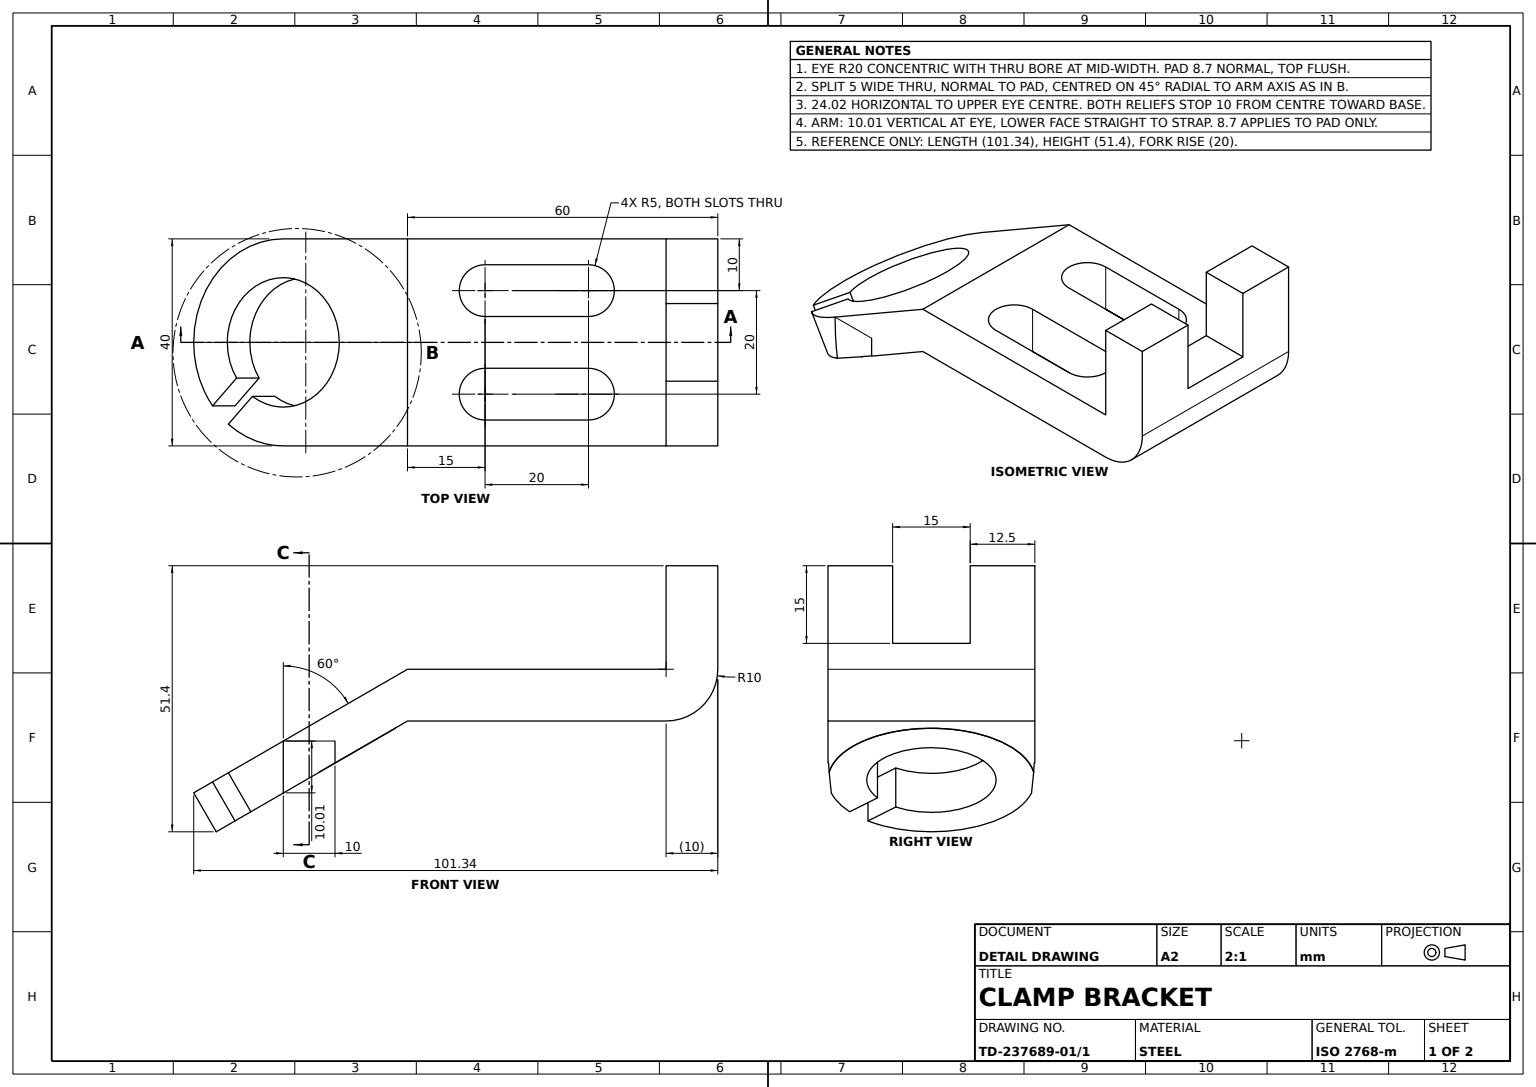
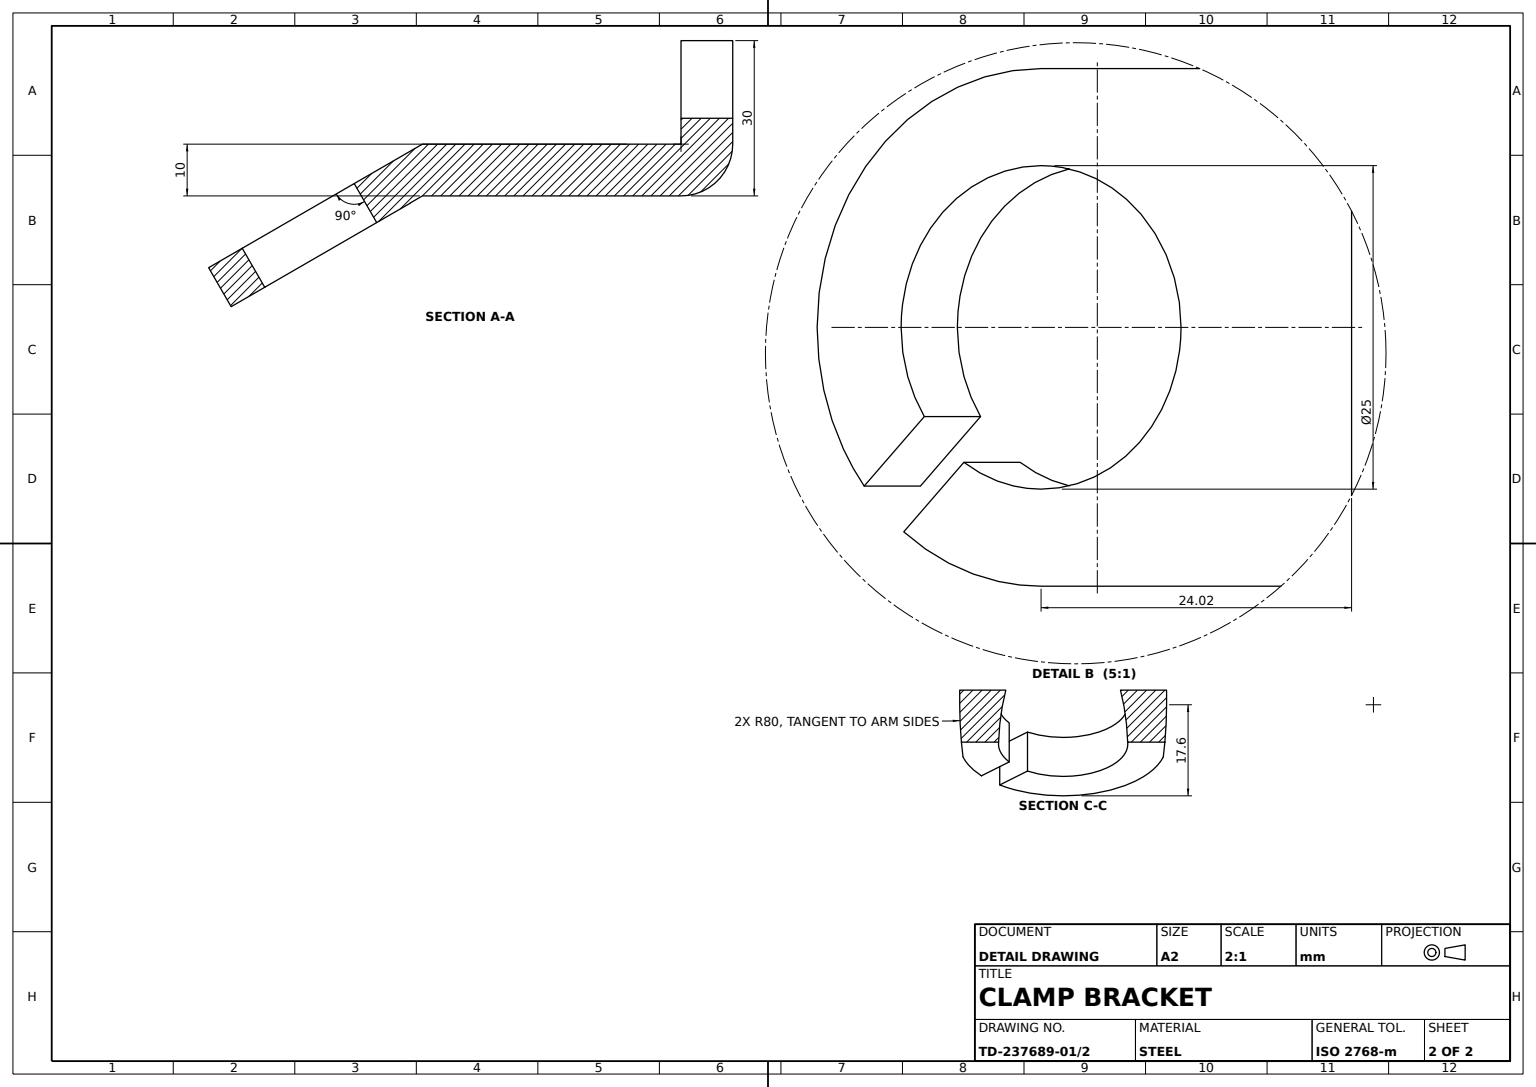
SolidWorks part; units mm, degrees
material "Plain Carbon Steel"
ref_plane "Front Plane" through (0, 0, 0) normal (0, 0, 1) x (1, 0, 0)
ref_plane "Top Plane" through (0, 0, 0) normal (0, 1, 0) x (1, 0, 0)
ref_plane "Right Plane" through (0, 0, 0) normal (1, 0, 0) x (0, 0, -1)
sketch "L-Profile Sketch" plane through (0, 0, 0) normal (0, 0, 1) x (1, 0, 0)
  line L0 (0, 0) -> (50, 0)
  line L1 (60, 10) -> (60, 30)
  line L2 (60, 30) -> (50, 30)
  line L3 (0, 0) -> (0, 10)
  line L4 (0, 10) -> (50, 10)
  line L5 (50, 10) -> (50, 30)
  arc A0 (50, 0) -> (60, 10) centre (50, 10) ccw
  point P6 (60, 0)
  dimension "D3" = 10
  dimension "D1" = 60
  dimension "D2" = 30
  dimension "D4" = 10
  dimension "D5" = 10
extrude "L-Bracket Base" add sketch "L-Profile Sketch" against normal blind 40
sketch "Corner Notch Sketch" plane through (50, 0, 0) normal (-1, 0, 0) x (0, 0, 1)
  line L0 (-27.5, 30) -> (-12.5, 30)
  line L1 (-40, 30) -> (0, 30) construction
  line L2 (-27.5, 30) -> (-27.5, 15)
  line L3 (-27.5, 15) -> (-12.5, 15)
  line L4 (-12.5, 15) -> (-12.5, 30)
  line L5 (-40, 30) -> (-40, 10) construction
  dimension "D1" = 12.5
  dimension "D2" = 15
  dimension "D3" = 15
extrude "Corner Notch" cut sketch "Corner Notch Sketch" against normal blind 40
sketch "Angled Arm Sketch 60deg" plane through (0, 0, 0) normal (0, 0, 1) x (1, 0, 0)
  line L1 (0, 10) -> (-24.0166, -3.866)
  line L3 (0, 10) -> (-24.0166, -3.866)
  line L5 (0, 0) -> (-24.0166, -13.8747)
  line L8 (0, 10) -> (0, 0) construction
  line L10 (-24.0166, -13.8747) -> (-24.0166, -3.866)
  line M2 (0, 10) -> (0, 0)
  dimension "D1" = 60
  dimension "D2" = 10.0087
  dimension "D3" = 24.0166
extrude "Angled Eye Arm" add sketch "Angled Arm Sketch 60deg" against normal blind 40 contours L10 L5 L1 M2
sketch "Eye Pad Sketch" plane through (-4.3301, 7.5, 0) normal (-0.5, 0.866, 0) x (0.866, 0.5, 0)
  line L0 (-22.7319, 40) -> (-22.7319, 0) construction
  circle A0 centre (-22.7319, 20) radius 20
  dimension "D1" = 40
extrude "Eye Pad" add sketch "Eye Pad Sketch" against normal blind 8.7
sketch "Slot 1 Sketch" plane through (-24.0166, 0, 0) normal (-1, 0, 0) x (0, 0, 1)
  line L0 (-0.6362, -13.8747) -> (0, -13.8747)
  line L1 (0, -13.8747) -> (0, -3.866)
  line L2 (0, -13.8747) -> (0, -3.866) construction
  arc A0 (0, -3.866) -> (-0.6362, -13.8747) centre (-80, -3.8053) cw
  ellipse E0 centre (-20, -3.866) end of major axis (0, -3.866) minor radius 10 (-40, -3.866) -> (0, -3.866) ccw construction
  dimension "D1" = 80
extrude "Slot 1" cut sketch "Slot 1 Sketch" against normal blind 10
sketch "Slot 2 Sketch" plane through (-24.0166, 0, 0) normal (-1, 0, 0) x (0, 0, 1)
  line L0 (-40, -13.8747) -> (-40, -3.866)
  line L1 (-40, -13.8747) -> (-39.3638, -13.8747)
  arc A0 (-39.3638, -13.8747) -> (-40, -3.866) centre (40, -3.8053) cw
  dimension "D1" = 80
extrude "Slot 2" cut sketch "Slot 2 Sketch" against normal blind 10
sketch "Split Eye Sketch" plane through (-4.3301, 7.5, 0) normal (-0.5, 0.866, 0) x (0.866, 0.5, 0)
  line L3 (-38.5309, 7.7366) -> (-33.1599, 13.1075)
  line L5 (-29.6244, 9.572) -> (-34.9954, 4.201)
  arc A0 (-29.6244, 9.572) -> (-33.1599, 13.1075) centre (-22.7319, 20) ccw
  arc A1 (-38.5309, 7.7366) -> (-34.9954, 4.201) centre (-22.7319, 20) ccw
  arc A2 (-22.7319, 40) -> (-22.7319, 0) centre (-22.7319, 20) ccw construction
  dimension "D1" = 25
  dimension "D5" = 40
  dimension "D2" = 5.371
  dimension "D3" = 5.371
  dimension "D4" = 6.8925
  dimension "D6" = 10.428
extrude "Split Eye Cut" cut sketch "Split Eye Sketch" against normal blind 10
sketch "U-Fork Sketch" plane through (0, 10, 0) normal (0, 1, 0) x (1, 0, 0)
  line L0 (50, 20) -> (0, 20)
  line L1 (50, 40) -> (50, 0) construction
  line L2 (0, 40) -> (0, 0) construction
  line L3 (15, 35) -> (35, 35)
  line L4 (15, 25) -> (35, 25)
  line L5 (15, 15) -> (35, 15)
  line L6 (15, 5) -> (35, 5)
  arc A0 (15, 35) -> (15, 25) centre (15, 30) ccw
  arc A1 (35, 25) -> (35, 35) centre (35, 30) ccw
  arc A2 (15, 15) -> (15, 5) centre (15, 10) ccw
  arc A3 (35, 5) -> (35, 15) centre (35, 10) ccw
  dimension "D1" = 10
  dimension "D2" = 10
  dimension "D7" = 10
  dimension "D8" = 10
  dimension "D3" = 15
  dimension "D4" = 10
  dimension "D5" = 10
  dimension "D6" = 20
  dimension "D9" = 10
  dimension "D10" = 15
  dimension "D11" = 10
  dimension "D12" = 20
extrude "U-Fork Cut" cut sketch "U-Fork Sketch" against normal blind 10 contours L4 A1 L3 A0 | L6 A3 L5 A2
